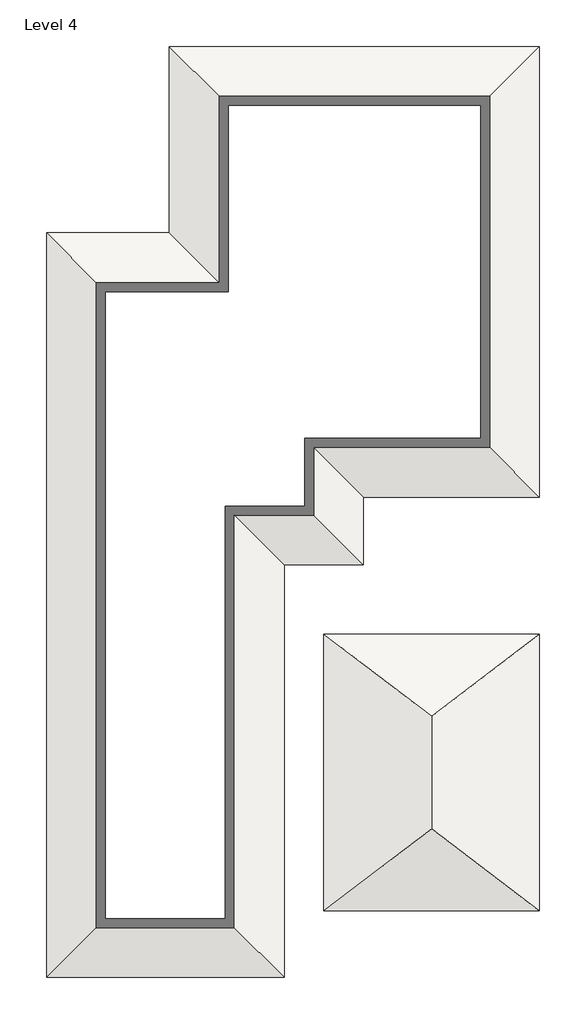
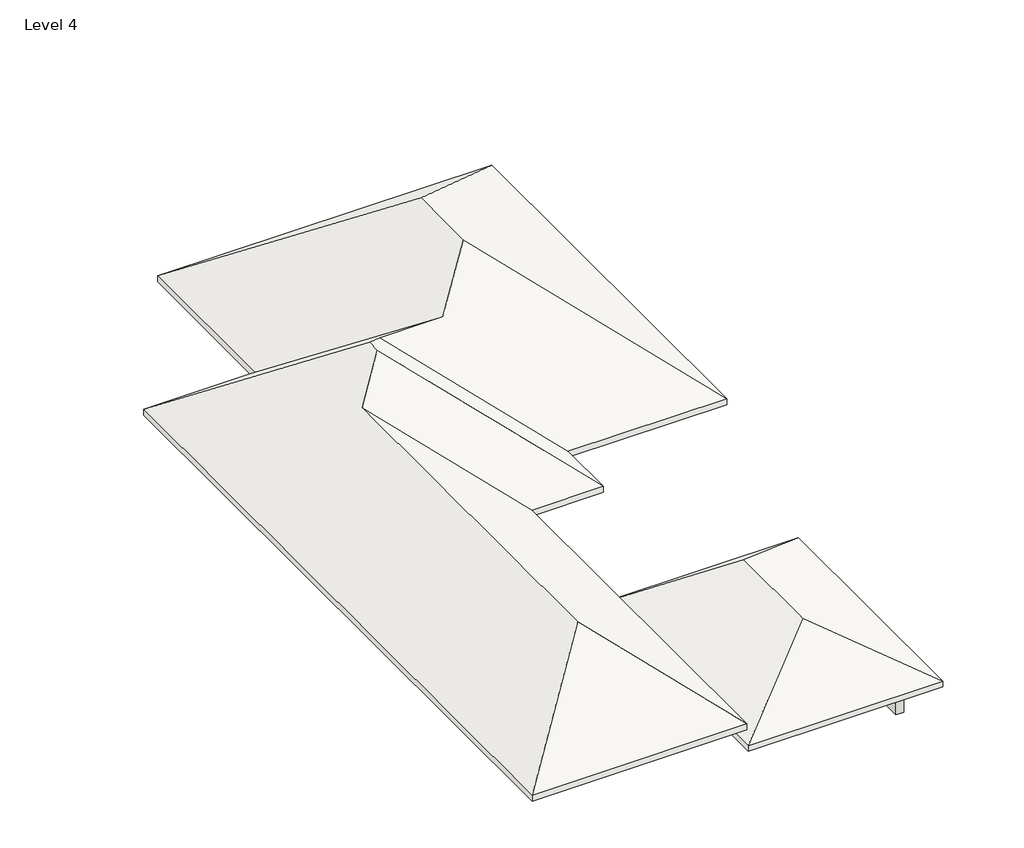
# One storey: 2 roofs, 1 wall.
"""IFC4 building model written with IfcOpenShell, lengths in millimetres."""

from ifc_helpers import new_model, si_unit, origin, place, context, project, spatial, faceted_brep, element, save

model = new_model("IFC4")

# Units and contexts
model_context = context("Model", 3, world=origin())
ifc_project = project(units=[si_unit("LENGTHUNIT", "METRE", prefix="MILLI")], contexts=[model_context])

# Site, building, storey
site = spatial("IfcSite", under=ifc_project)
building = spatial("IfcBuilding", under=site)
storey = spatial("IfcBuildingStorey", under=building, Name="Level 4", Elevation=6858.0)

# Roofs
placement = place(None, origin())
element("IfcRoof", 1, ObjectType="roof 6\"", at=placement, inside=storey, context=model_context, shape_type="Brep", body=[
    faceted_brep([(-725.1403048, -1607.6444793, 6858.0), (-5716.2403048, 3383.4555207, 10601.325), (-5716.2403048, 5555.1555207, 10601.325), (-725.1403048, 10546.2555207, 6858.0), (-10707.3403048, 10546.2555207, 6858.0), (-7144.9903048, 1954.7055207, 9529.7625), (-10707.3403048, 5517.0555207, 6858.0), (-14020.6629606, -14564.1978416, 6858.0), (-10813.9902635, -11357.5251445, 9263.0045228), (-7607.3175664, -14564.1978416, 6858.0), (-5473.7175664, -3436.4444793, 6858.0), (-9747.1902635, 837.0282178, 10063.1045228), (-9747.1902635, 1243.5828236, 10063.1045228), (-9036.0675664, 1954.7055207, 9529.7625), (-5473.7175664, -1607.6444793, 6858.0), (-14020.6629606, 5517.0555207, 6858.0), (-10813.9902635, -229.7717822, 9263.0045228), (-7607.3175664, -3436.4444793, 6858.0), (-725.1403048, -1607.6444793, 7048.5), (-725.1403048, 10546.2555207, 7048.5), (-5716.2403048, 5555.1555207, 10791.825), (-5716.2403048, 3383.4555207, 10791.825), (-10707.3403048, 10546.2555207, 7048.5), (-10707.3403048, 5517.0555207, 7048.5), (-7144.9903048, 1954.7055207, 9720.2625), (-14020.6629606, -14564.1978416, 7048.5), (-7607.3175664, -14564.1978416, 7048.5), (-10813.9902635, -11357.5251445, 9453.5045228), (-5473.7175664, -3436.4444793, 7048.5), (-5473.7175664, -1607.6444793, 7048.5), (-9036.0675664, 1954.7055207, 9720.2625), (-9747.1902635, 1243.5828236, 10253.6045228), (-9747.1902635, 837.0282178, 10253.6045228), (-14020.6629606, 5517.0555207, 7048.5), (-10813.9902635, -229.7717822, 9453.5045228), (-7607.3175664, -3436.4444793, 7048.5)], [[[0, 1, 2, 3]], [[3, 2, 4]], [[4, 2, 1, 5, 6]], [[7, 8, 9]], [[10, 11, 12, 13, 14]], [[15, 12, 11, 16, 8, 7]], [[0, 14, 13, 5, 1]], [[9, 8, 16, 17]], [[6, 5, 13, 12, 15]], [[17, 16, 11, 10]], [[18, 19, 20, 21]], [[19, 22, 20]], [[22, 23, 24, 21, 20]], [[25, 26, 27]], [[28, 29, 30, 31, 32]], [[33, 25, 27, 34, 32, 31]], [[18, 21, 24, 30, 29]], [[26, 35, 34, 27]], [[23, 33, 31, 30, 24]], [[35, 28, 32, 34]], [[3, 19, 18, 0]], [[4, 22, 19, 3]], [[6, 23, 22, 4]], [[15, 33, 23, 6]], [[7, 25, 33, 15]], [[9, 26, 25, 7]], [[17, 35, 26, 9]], [[10, 28, 35, 17]], [[14, 29, 28, 10]], [[0, 18, 29, 14]]]),
])
element("IfcRoof", 2, ObjectType="roof 6\"", at=placement, inside=storey, context=model_context, shape_type="Brep", body=[
    faceted_brep([(-6537.4131952, -12751.1254401, 4724.4), (-3631.27675, -10531.3532174, 6389.2291671), (-725.1403048, -12751.1254401, 4724.4), (-3631.27675, -7542.9357412, 6389.2291671), (-725.1403048, -5323.1635184, 4724.4), (-6537.4131952, -5323.1635184, 4724.4), (-6537.4131952, -12770.9444793, 4900.0357206), (-725.1403048, -12770.9444793, 4900.0357206), (-3631.27675, -10551.1722565, 6564.8648877), (-725.1403048, -5303.3444793, 4900.0357206), (-3631.27675, -7523.1167021, 6564.8648877), (-6537.4131952, -5303.3444793, 4900.0357206), (-725.1403048, -12770.9444793, 4724.4), (-6537.4131952, -12770.9444793, 4724.4), (-725.1403048, -5303.3444793, 4724.4), (-6537.4131952, -5303.3444793, 4724.4)], [[[0, 1, 2]], [[2, 1, 3, 4]], [[1, 0, 5, 3]], [[4, 3, 5]], [[6, 7, 8]], [[7, 9, 10, 8]], [[6, 8, 10, 11]], [[9, 11, 10]], [[12, 7, 6, 13]], [[14, 9, 7, 12, 2, 4]], [[15, 11, 9, 14]], [[13, 6, 11, 15, 5, 0]], [[13, 0, 2, 12]], [[5, 15, 14, 4]]]),
])

# Wall
element("IfcWall", 3, ObjectType="9\" wall", at=placement, inside=storey, context=model_context, shape_type="Brep", body=[
    faceted_brep([(-1410.9403048, -11932.7444793, 3657.6), (-1410.9403048, -5341.4444793, 3657.6), (-1410.9403048, -5341.4444793, 3810.0), (-1410.9403048, -5341.4444793, 4738.1107206), (-1410.9403048, -5846.992946, 5117.2720706), (-1410.9403048, -11932.7444793, 5117.2720706), (-1410.9403048, -11932.7444793, 4114.8), (-1410.9403048, -11932.7444793, 3810.0), (-1639.5403048, -11932.7444793, 3657.6), (-1639.5403048, -11932.7444793, 5248.2294275), (-1639.5403048, -6021.6027551, 5248.2294275), (-1639.5403048, -5341.4444793, 4738.1107206), (-1639.5403048, -5341.4444793, 3810.0), (-1639.5403048, -5341.4444793, 3657.6)], [[[0, 1, 2, 3, 4, 5, 6, 7]], [[8, 9, 10, 11, 12, 13]], [[1, 0, 8, 13]], [[3, 2, 1, 13, 12, 11]], [[0, 7, 6, 5, 9, 8]], [[5, 4, 10, 9]], [[4, 3, 11, 10]]]),
])

save(model, "model.ifc")

# Revit data of these elements
# Type "roof 6\""
#   Assembly Code = "B1020"
#   Layers, outside or top first: 0' - 6" "ROOF" (function 1)
# Type "9\" wall"
#   Assembly Code = "B2010"
# Element 1 (IfcRoof, "roof 6\"")
#   built-in parameter 1001705 = 35.4063 (stored number, unit not read)
#   built-in parameter 1001710 = 33615
#   Phase Created = New Construction
#   Materials on its faces: "ROOF"
# Element 2 (IfcRoof, "roof 6\"")
#   built-in parameter 1001705 = 21.5383 (stored number, unit not read)
#   built-in parameter 1001701 = -7 (stored number, unit not read)
#   built-in parameter 1001710 = 33615
#   Phase Created = New Construction
#   Materials on its faces: "ROOF"
# Element 3 (IfcWall, "9\" wall")
#   built-in parameter 1001111 = -10' - 6"
#   Top Offset = -9' - 7.70426"
#   Base Offset = -10' - 6"
#   wall height = 1' - 4.29574"
#   Phase Created = New Construction
#   Base Constraint = Level 4
#   Top Constraint = Level 5
# Materials
#   "ROOF": class "Generic", colour RGB 120 120 120, transparency 0, Cost = 0
